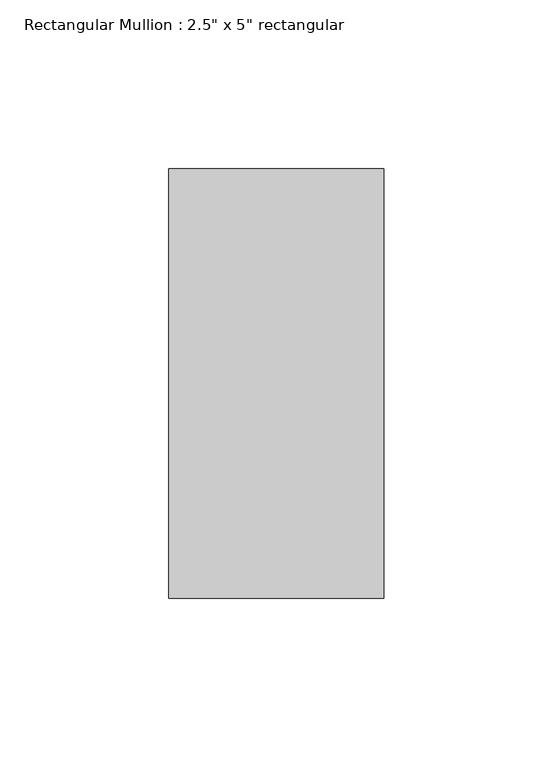
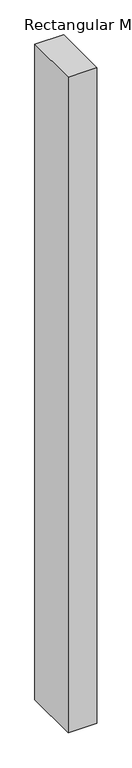
"""IFC4 building model written with IfcOpenShell, lengths in millimetres: member geometry."""

from ifc_helpers import new_model, si_unit, frame, origin, place, context, project, spatial, polyline, outline, extrude, source, transform, mapped, element, save


def member_72fd50dd(model_context):
    return source(origin(), model_context, "Body", "SweptSolid", [
        extrude(outline(polyline([(0.0, 63.5), (0.0, -63.5), (-63.5, -63.5), (-63.5, 63.5), (0.0, 63.5)])), frame((0.0, 0.0, -1531.3368617), z_axis=(0.0, 0.0, 1.0), x_axis=(1.0, 0.0, 0.0)), (0.0, 0.0, 1.0), 1531.3368617),
    ])


if __name__ == "__main__":
    model = new_model("IFC4")
    model_context = context("Model", 3, world=origin())
    ifc_project = project(units=[si_unit("LENGTHUNIT", "METRE", prefix="MILLI")], contexts=[model_context])
    site = spatial("IfcSite", under=ifc_project)
    building = spatial("IfcBuilding", under=site)
    placement = place(None, origin())
    member_shape = member_72fd50dd(model_context)
    element("IfcMember", 1, ObjectType="Rectangular Mullion : 2.5\" x 5\" rectangular", at=placement, inside=building, context=model_context, shape_type="MappedRepresentation", body=[
        mapped(member_shape, transform((0.0, 0.0, 0.0), x_axis=(1.0, 0.0, 0.0), y_axis=(0.0, 1.0, 0.0), z_axis=(0.0, 0.0, 1.0))),
    ])
    save(model, "model.ifc")

# Revit data of these elements
# Type "Rectangular Mullion : 2.5\" x 5\" rectangular"
#   built-in parameter 1007304 = 0.416667 (stored number, unit not read)
#   built-in parameter 1007301 = 0.104167 (stored number, unit not read)
#   built-in parameter 1007300 = 0.104167 (stored number, unit not read)
# Element 1 (IfcMember, "Rectangular Mullion : 2.5\" x 5\" rectangular")
#   Materials on its faces: "Aluminum"
# Materials
#   "Aluminum": class "Metal", colour RGB 247 247 247, transparency 0, Description = "Aluminum 6061", Cost = 0
